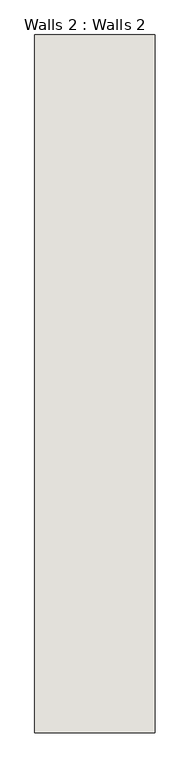
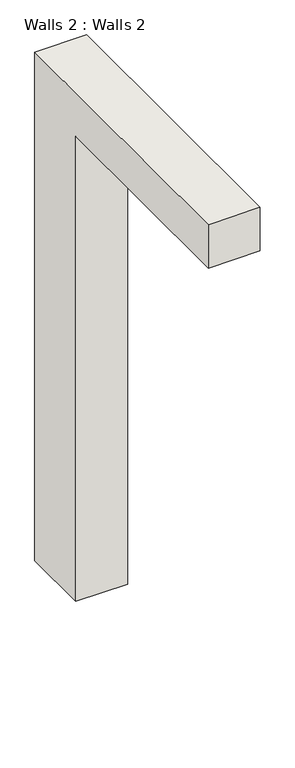
"""IFC4 building model written with IfcOpenShell, lengths in millimetres: wall geometry, Walls 2 : Walls 2."""

from ifc_helpers import new_model, si_unit, frame, origin, place, context, project, spatial, polyline, outline, extrude, source, transform, mapped, element, save


def walls_2_walls_2_b5bda089(model_context):
    return source(origin(), model_context, "Body", "SweptSolid", [
        extrude(outline(polyline([(-1845.8046854, 2762.6009455), (-1845.8046854, 0.0), (-2210.3056457, 0.0), (-2210.3056457, 2525.7941791), (-3390.9180898, 2525.7941791), (-3390.9180898, 2762.6009455), (-1845.8046854, 2762.6009455)])), frame((-16064.8955662, 0.0, 0.0), z_axis=(1.0, 0.0, 0.0), x_axis=(0.0, 1.0, 0.0)), (0.0, 0.0, 1.0), 266.2058338),
    ])


if __name__ == "__main__":
    model = new_model("IFC4")
    model_context = context("Model", 3, world=origin())
    ifc_project = project(units=[si_unit("LENGTHUNIT", "METRE", prefix="MILLI")], contexts=[model_context])
    site = spatial("IfcSite", under=ifc_project)
    building = spatial("IfcBuilding", under=site)
    placement = place(None, origin())
    walls_2_walls_2_shape = walls_2_walls_2_b5bda089(model_context)
    element("IfcWall", 1, ObjectType="Walls 2 : Walls 2", at=placement, inside=building, context=model_context, shape_type="MappedRepresentation", body=[
        mapped(walls_2_walls_2_shape, transform((0.0, 0.0, 0.0), x_axis=(1.0, 0.0, 0.0), y_axis=(0.0, 1.0, 0.0), z_axis=(0.0, 0.0, 1.0))),
    ])
    save(model, "model.ifc")

# Revit data of these elements
# Element 1 (IfcWall, "Walls 2 : Walls 2")
#   Materials on its faces: "Default Wall"
# Materials
#   "Default Wall": colour RGB 80 80 80, transparency 0
